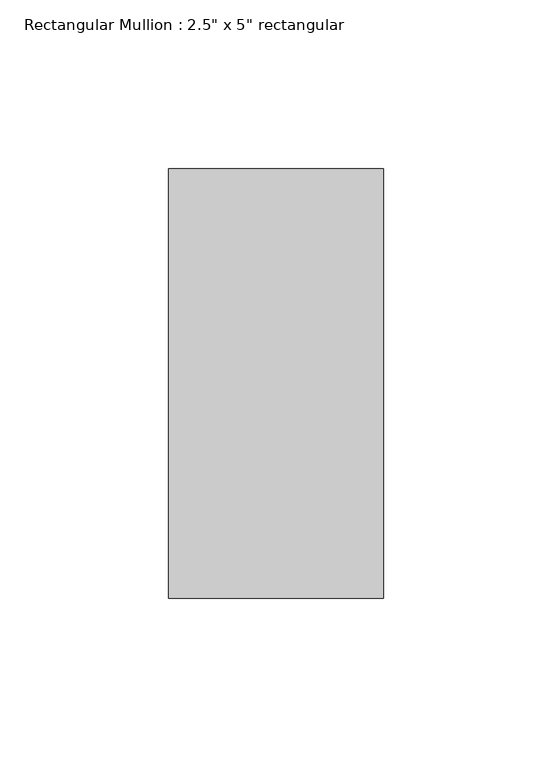
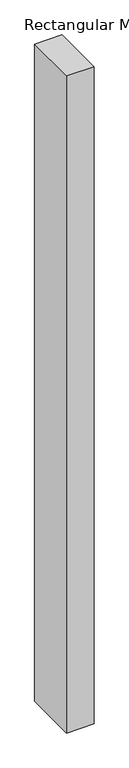
"""IFC4 building model written with IfcOpenShell, lengths in millimetres: member geometry."""

from ifc_helpers import new_model, si_unit, frame, origin, place, context, project, spatial, polyline, outline, extrude, source, transform, mapped, element, save


def member_693a6220(model_context):
    return source(origin(), model_context, "Body", "SweptSolid", [
        extrude(outline(polyline([(0.0, 63.5), (0.0, -63.5), (-63.5, -63.5), (-63.5, 63.5), (0.0, 63.5)])), frame((0.0, 0.0, -1602.5825326), z_axis=(0.0, 0.0, 1.0), x_axis=(1.0, 0.0, 0.0)), (0.0, 0.0, 1.0), 1602.5825326),
    ])


if __name__ == "__main__":
    model = new_model("IFC4")
    model_context = context("Model", 3, world=origin())
    ifc_project = project(units=[si_unit("LENGTHUNIT", "METRE", prefix="MILLI")], contexts=[model_context])
    site = spatial("IfcSite", under=ifc_project)
    building = spatial("IfcBuilding", under=site)
    placement = place(None, origin())
    member_shape = member_693a6220(model_context)
    element("IfcMember", 1, ObjectType="Rectangular Mullion : 2.5\" x 5\" rectangular", at=placement, inside=building, context=model_context, shape_type="MappedRepresentation", body=[
        mapped(member_shape, transform((0.0, 0.0, 0.0), x_axis=(1.0, 0.0, 0.0), y_axis=(0.0, 1.0, 0.0), z_axis=(0.0, 0.0, 1.0))),
    ])
    save(model, "model.ifc")

# Revit data of these elements
# Type "Rectangular Mullion : 2.5\" x 5\" rectangular"
#   built-in parameter 1007304 = 0.416667 (stored number, unit not read)
#   built-in parameter 1007301 = 0.104167 (stored number, unit not read)
#   built-in parameter 1007300 = 0.104167 (stored number, unit not read)
# Element 1 (IfcMember, "Rectangular Mullion : 2.5\" x 5\" rectangular")
#   Materials on its faces: "Aluminum"
# Materials
#   "Aluminum": class "Metal", colour RGB 247 247 247, transparency 0, Description = "Aluminum 6061", Cost = 0
